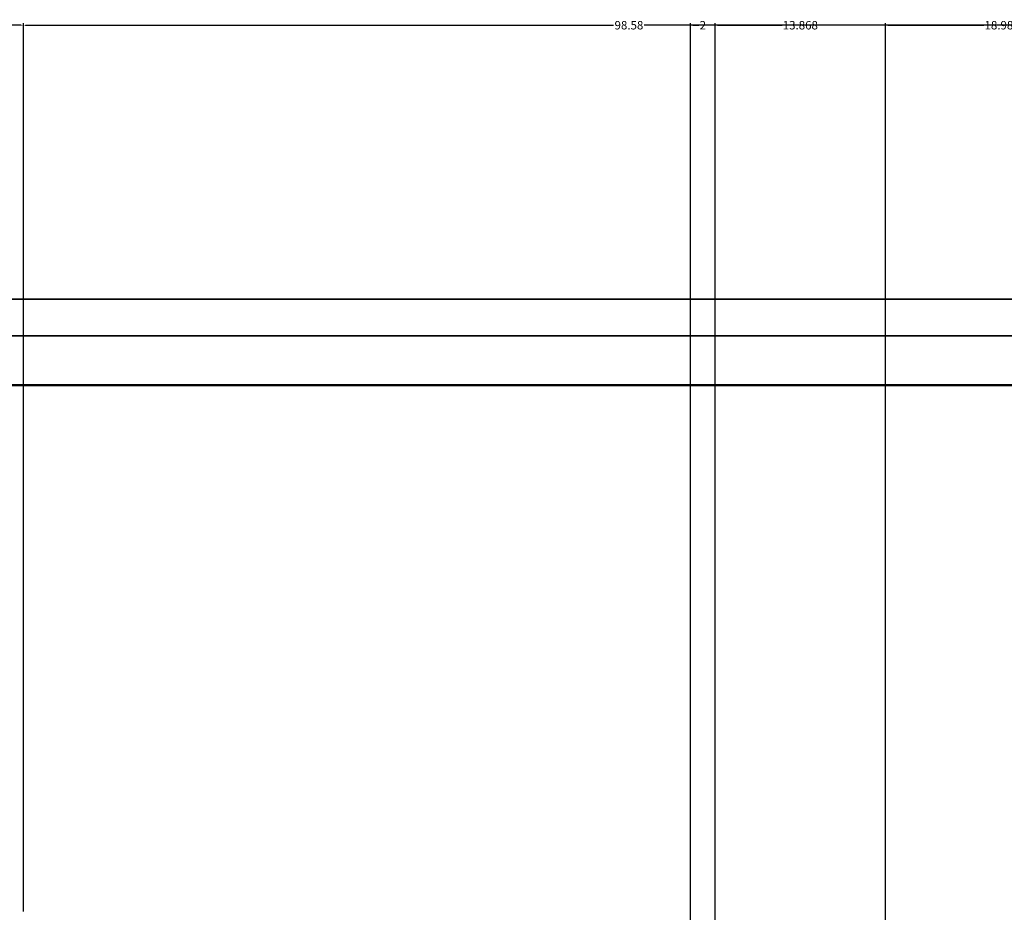
# Model space of a CAD drawing. Units: inches. Extents: x -139 to 346, y 72 to 413.
# Tile 16 of 18: x 175 to 256, y 340 to 413. Entities that reach past the tile are written whole.
import ezdxf

# ---------------------------------------------------------------- set-up
doc = ezdxf.new("R2010")
doc.units = ezdxf.units.IN
doc.header["$MEASUREMENT"] = 0
for name, color, linetype, lineweight in [('A-ANNO-DIMS', 2, 'Continuous', 18), ('A-ROOF', 1, 'Continuous', 35), ('A-WALL', 7, 'Continuous', 50)]:
    doc.layers.add(name, color=color, linetype=linetype, lineweight=lineweight)
doc.styles.get("Standard").update_dxf_attribs({"font": 'arial.ttf'})
doc.dimstyles.get("Standard").update_dxf_attribs({"dimtxt": 0.6875, "dimasz": 0.18, "dimexe": 0.18, "dimexo": 0.0625, "dimgap": 0.09, "dimtad": 0, "dimtih": 1, "dimtoh": 1, "dimdec": 4, "dimzin": 0, "dimdsep": 46, "dimlunit": 4, "dimtxsty": 'Standard', "dimcen": 0.09, "dimadec": 0, "dimazin": 0, "dimtfac": 1, "dimtdec": 4, "dimtofl": 0, "dimtmove": 0, "dimatfit": 3, "dimfxl": 1, "dimtolj": 1, "dimtzin": 0, "dimarcsym": 0})

# ---------------------------------------------------------------- blocks, each defined once
blk = doc.blocks.new('*D27')
at = {"layer": 'A-ANNO-DIMS', "color": 0, "lineweight": -2, "transparency": 16777216}
for p, q in [((112.651, 291.123), (112.651, 412.455)), ((112.831, 412.275), (142.911, 412.275)), ((175.488, 412.275), (145.407, 412.275)), ((175.668, 340.117), (175.668, 412.455))]:
    blk.add_line(p, q, dxfattribs=at)
at = {"layer": 'A-ANNO-DIMS', "color": 0, "transparency": 16777216}
for points in [[(112.831, 412.305), (112.831, 412.245), (112.651, 412.275)], [(175.488, 412.305), (175.488, 412.245), (175.668, 412.275)]]:
    blk.add_solid(points, dxfattribs=at)
at = {"layer": 'Defpoints', "color": 0, "transparency": 16777216}
for p in [(175.668, 412.275), (175.668, 340.055), (112.651, 291.06)]:
    blk.add_point(p, dxfattribs=at)
at = {"layer": 'A-ANNO-DIMS', "color": 0, "transparency": 16777216, "insert": (144.159, 412.275), "char_height": 0.6875, "attachment_point": 5}
blk.add_mtext('\\A1;63.02', dxfattribs=at)
blk = doc.blocks.new('*D28')
at = {"layer": 'A-ANNO-DIMS', "color": 0, "lineweight": -2, "transparency": 16777216}
for p, q in [((175.668, 340.117), (175.668, 412.455)), ((175.848, 412.275), (223.706, 412.275)), ((274.067, 412.275), (226.208, 412.275)), ((274.247, 340.117), (274.247, 412.455))]:
    blk.add_line(p, q, dxfattribs=at)
at = {"layer": 'A-ANNO-DIMS', "color": 0, "transparency": 16777216}
for points in [[(175.848, 412.305), (175.848, 412.245), (175.668, 412.275)], [(274.067, 412.305), (274.067, 412.245), (274.247, 412.275)]]:
    blk.add_solid(points, dxfattribs=at)
at = {"layer": 'Defpoints', "color": 0, "transparency": 16777216}
for p in [(274.247, 412.275), (175.668, 340.055), (274.247, 340.055)]:
    blk.add_point(p, dxfattribs=at)
at = {"layer": 'A-ANNO-DIMS', "color": 0, "transparency": 16777216, "insert": (224.957, 412.275), "char_height": 0.6875, "attachment_point": 5}
blk.add_mtext('\\A1;98.58', dxfattribs=at)
blk = doc.blocks.new('*D80')
at = {"layer": 'A-ANNO-DIMS', "color": 0, "lineweight": -2, "transparency": 16777216}
for p, q in [((229.972, 205.587), (229.972, 412.455)), ((230.152, 412.275), (230.654, 412.275)), ((231.792, 412.275), (231.29, 412.275)), ((231.972, 203.587), (231.972, 412.455))]:
    blk.add_line(p, q, dxfattribs=at)
at = {"layer": 'A-ANNO-DIMS', "color": 0, "transparency": 16777216}
for points in [[(230.152, 412.305), (230.152, 412.245), (229.972, 412.275)], [(231.792, 412.305), (231.792, 412.245), (231.972, 412.275)]]:
    blk.add_solid(points, dxfattribs=at)
at = {"layer": 'Defpoints', "color": 0, "transparency": 16777216}
for p in [(231.972, 412.275), (229.972, 205.524), (231.972, 203.524)]:
    blk.add_point(p, dxfattribs=at)
at = {"layer": 'A-ANNO-DIMS', "color": 0, "transparency": 16777216, "insert": (230.972, 412.275), "char_height": 0.6875, "attachment_point": 5}
blk.add_mtext('\\A1;2', dxfattribs=at)
blk = doc.blocks.new('*D81')
at = {"layer": 'A-ANNO-DIMS', "color": 0, "lineweight": -2, "transparency": 16777216}
for p, q in [((231.972, 203.587), (231.972, 412.455)), ((232.152, 412.275), (237.421, 412.275)), ((245.66, 412.275), (240.391, 412.275)), ((245.84, 184.668), (245.84, 412.455))]:
    blk.add_line(p, q, dxfattribs=at)
at = {"layer": 'A-ANNO-DIMS', "color": 0, "transparency": 16777216}
for points in [[(232.152, 412.305), (232.152, 412.245), (231.972, 412.275)], [(245.66, 412.305), (245.66, 412.245), (245.84, 412.275)]]:
    blk.add_solid(points, dxfattribs=at)
at = {"layer": 'Defpoints', "color": 0, "transparency": 16777216}
for p in [(245.84, 412.275), (231.972, 203.524), (245.84, 184.606)]:
    blk.add_point(p, dxfattribs=at)
at = {"layer": 'A-ANNO-DIMS', "color": 0, "transparency": 16777216, "insert": (238.906, 412.275), "char_height": 0.6875, "attachment_point": 5}
blk.add_mtext('\\A1;13.868', dxfattribs=at)
blk = doc.blocks.new('*D82')
at = {"layer": 'A-ANNO-DIMS', "color": 0, "lineweight": -2, "transparency": 16777216}
for p, q in [((245.84, 184.668), (245.84, 412.455)), ((246.02, 412.275), (253.85, 412.275)), ((264.642, 412.275), (256.812, 412.275)), ((264.822, 184.668), (264.822, 412.455))]:
    blk.add_line(p, q, dxfattribs=at)
at = {"layer": 'A-ANNO-DIMS', "color": 0, "transparency": 16777216}
for points in [[(246.02, 412.305), (246.02, 412.245), (245.84, 412.275)], [(264.642, 412.305), (264.642, 412.245), (264.822, 412.275)]]:
    blk.add_solid(points, dxfattribs=at)
at = {"layer": 'Defpoints', "color": 0, "transparency": 16777216}
for p in [(264.822, 412.275), (245.84, 184.606), (264.822, 184.606)]:
    blk.add_point(p, dxfattribs=at)
at = {"layer": 'A-ANNO-DIMS', "color": 0, "transparency": 16777216, "insert": (255.331, 412.275), "char_height": 0.6875, "attachment_point": 5}
blk.add_mtext('\\A1;18.982', dxfattribs=at)

msp = doc.modelspace()

# ---------------------------------------------------------------- linework, layer by layer
at = {"layer": 'A-ROOF'}
for p, q in [((-47.2734, 389.9748), (309.8894, 389.9748)), ((-47.2734, 386.9748), (309.8894, 386.9748))]:
    msp.add_line(p, q, dxfattribs=at)
at = {"layer": 'A-WALL'}
msp.add_line((309.8894, 382.9748), (89.4597, 382.9748), dxfattribs=at)

# ---------------------------------------------------------------- dimensions: what is measured, and where the dimension line sits
at = {"layer": 'A-ANNO-DIMS'}
for base, p1, p2, override, picture, middle in [((175.6676, 412.2748), (112.6506, 291.0604), (175.6676, 340.0548), {"dimdec": 2, "dimlfac": 1, "dimrnd": 0, "dimzin": 0, "dimdsep": 46, "dimlunit": 2}, '*D27', (144.1591, 412.2748)), ((274.2465, 412.2748), (175.6676, 340.0548), (274.2465, 340.0548), {"dimdec": 2, "dimlfac": 1, "dimrnd": 0, "dimzin": 0, "dimdsep": 46, "dimlunit": 2}, '*D28', (224.957, 412.2748)), ((231.972, 412.2748), (229.972, 205.5243), (231.972, 203.5243), {"dimdec": 0, "dimlfac": 1, "dimrnd": 0, "dimzin": 0, "dimdsep": 46, "dimlunit": 2}, '*D80', (230.972, 412.2748)), ((245.8399, 412.2748), (231.972, 203.5243), (245.8399, 184.6055), {"dimdec": 3, "dimlfac": 1, "dimrnd": 0, "dimzin": 0, "dimdsep": 46, "dimlunit": 2}, '*D81', (238.906, 412.2748)), ((264.8219, 412.2748), (245.8399, 184.6055), (264.8219, 184.6055), {"dimdec": 3, "dimlfac": 1, "dimrnd": 0, "dimzin": 0, "dimdsep": 46, "dimlunit": 2}, '*D82', (255.3309, 412.2748))]:
    dim = msp.add_linear_dim(base=base, p1=p1, p2=p2, dimstyle='Standard', override=override, dxfattribs=at)
    dim.commit()
    dim.dimension.update_dxf_attribs({"geometry": picture, "text_midpoint": middle})

doc.saveas('drawing.dxf')
